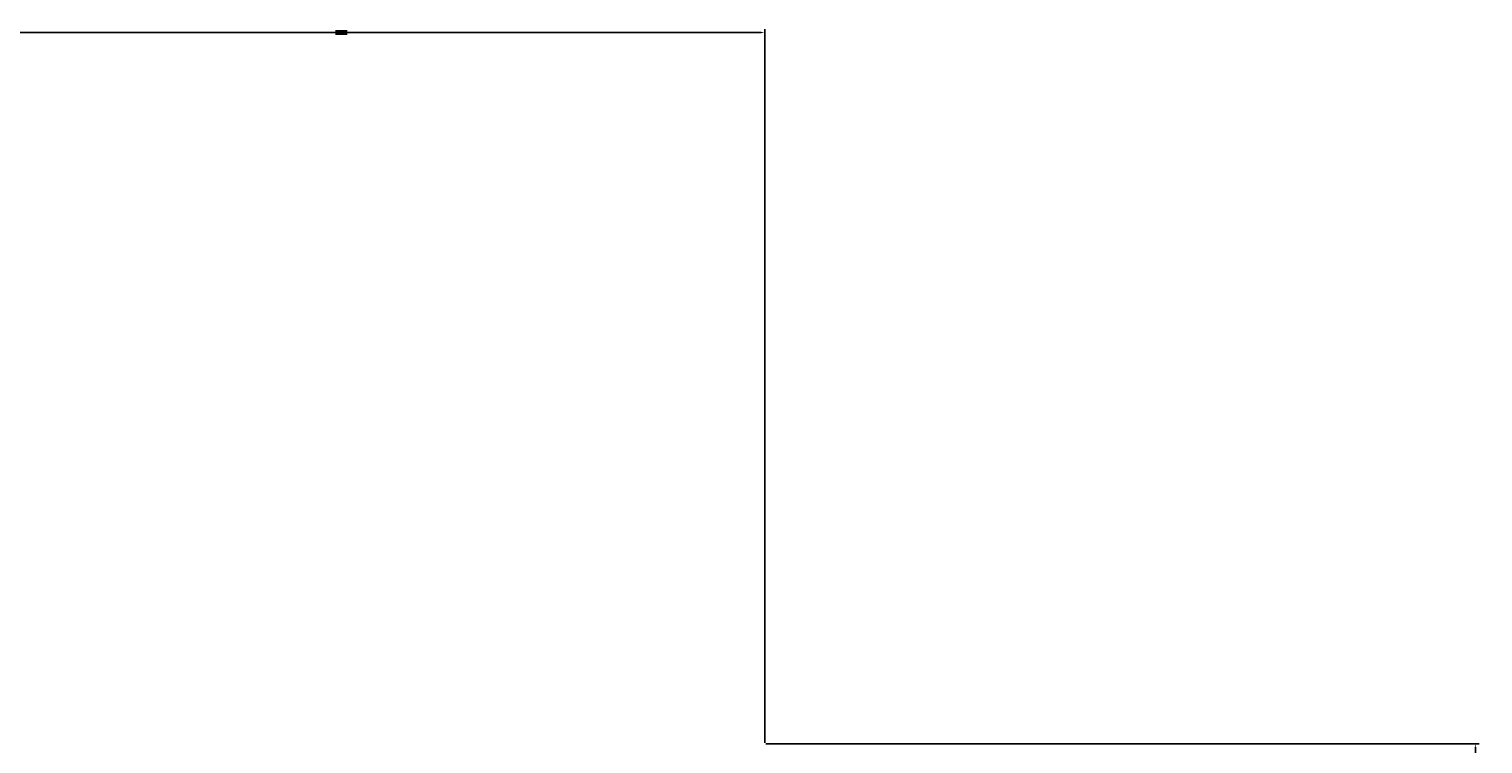
# Model space of a CAD drawing. Units: inches. Extents: x -128 to 854, y -395 to 398.
# Tile 50 of 61: x 275 to 352, y 349 to 387. Entities that reach past the tile are written whole.
import ezdxf

# ---------------------------------------------------------------- set-up
doc = ezdxf.new("R2010")
doc.units = ezdxf.units.IN
doc.header["$MEASUREMENT"] = 0
doc.layers.add('A-ANNO-DIMS', color=2, linetype='Continuous', lineweight=18)
doc.styles.get("Standard").update_dxf_attribs({"font": 'arial.ttf'})
doc.dimstyles.get("Standard").update_dxf_attribs({"dimtxt": 0.18, "dimasz": 0.18, "dimexe": 0.18, "dimexo": 0.0625, "dimgap": 0.09, "dimtad": 0, "dimtih": 1, "dimtoh": 1, "dimdec": 1, "dimzin": 0, "dimdsep": 46, "dimlunit": 4, "dimtxsty": 'Standard', "dimcen": 0.09, "dimclrd": 1, "dimclre": 2, "dimclrt": 6, "dimadec": 0, "dimazin": 0, "dimtfac": 1, "dimtdec": 1, "dimtofl": 0, "dimtmove": 0, "dimatfit": 3, "dimfxl": 1, "dimtfill": 2, "dimtfillclr": 3, "dimtolj": 1, "dimtzin": 0, "dimarcsym": 0})

# ---------------------------------------------------------------- blocks, each defined once
blk = doc.blocks.new('*D97')
at = {"layer": 'A-ANNO-DIMS', "color": 2, "lineweight": -2, "transparency": 16777216}
for p, q in [((-50.127, 348.803), (-50.127, 386.743)), ((313.873, 348.803), (313.873, 386.743))]:
    blk.add_line(p, q, dxfattribs=at)
at = {"layer": 'A-ANNO-DIMS', "color": 1, "lineweight": -2, "transparency": 16777216}
for p, q in [((-49.947, 386.563), (131.474, 386.563)), ((313.693, 386.563), (132.272, 386.563))]:
    blk.add_line(p, q, dxfattribs=at)
at = {"layer": 'A-ANNO-DIMS', "color": 1, "transparency": 16777216}
for points in [[(-49.947, 386.593), (-49.947, 386.533), (-50.127, 386.563)], [(313.693, 386.593), (313.693, 386.533), (313.873, 386.563)]]:
    blk.add_solid(points, dxfattribs=at)
at = {"layer": 'Defpoints', "color": 0, "transparency": 16777216}
for p in [(313.873, 386.563), (-50.127, 348.741), (313.873, 348.741)]:
    blk.add_point(p, dxfattribs=at)
at = {"layer": 'A-ANNO-DIMS', "color": 6, "transparency": 16777216, "insert": (131.873, 386.563), "char_height": 0.18, "attachment_point": 5, "bg_fill": 1, "box_fill_scale": 1.25, "bg_fill_color": 3, "bg_fill_transparency": 0}
blk.add_mtext('\\A1;30\'-4"', dxfattribs=at)
blk = doc.blocks.new('*D98')
at = {"layer": 'A-ANNO-DIMS', "color": 2, "lineweight": -2, "transparency": 16777216}
for p, q in [((313.935, 348.741), (351.853, 348.741)), ((313.935, -89.259), (351.853, -89.259))]:
    blk.add_line(p, q, dxfattribs=at)
at = {"layer": 'A-ANNO-DIMS', "color": 1, "lineweight": -2, "transparency": 16777216}
for p, q in [((351.673, 348.561), (351.673, 129.923)), ((351.673, -89.079), (351.673, 129.559))]:
    blk.add_line(p, q, dxfattribs=at)
at = {"layer": 'A-ANNO-DIMS', "color": 1, "transparency": 16777216}
for points in [[(351.643, 348.561), (351.703, 348.561), (351.673, 348.741)], [(351.643, -89.079), (351.703, -89.079), (351.673, -89.259)]]:
    blk.add_solid(points, dxfattribs=at)
at = {"layer": 'Defpoints', "color": 0, "transparency": 16777216}
for p in [(313.873, 348.741), (351.673, 348.741), (313.873, -89.259)]:
    blk.add_point(p, dxfattribs=at)
at = {"layer": 'A-ANNO-DIMS', "color": 6, "transparency": 16777216, "insert": (351.673, 129.741), "char_height": 0.18, "attachment_point": 5, "bg_fill": 1, "box_fill_scale": 1.25, "bg_fill_color": 3, "bg_fill_transparency": 0}
blk.add_mtext('\\A1;36\'-6"', dxfattribs=at)
blk = doc.blocks.new('*D105')
at = {"layer": 'A-ANNO-DIMS', "color": 2, "lineweight": -2, "transparency": 16777216}
for p, q in [((268.873, 348.803), (268.873, 386.743)), ((313.873, 348.803), (313.873, 386.743))]:
    blk.add_line(p, q, dxfattribs=at)
at = {"layer": 'A-ANNO-DIMS', "color": 1, "lineweight": -2, "transparency": 16777216}
for p, q in [((269.053, 386.563), (291.044, 386.563)), ((313.693, 386.563), (291.702, 386.563))]:
    blk.add_line(p, q, dxfattribs=at)
at = {"layer": 'A-ANNO-DIMS', "color": 1, "transparency": 16777216}
for points in [[(269.053, 386.593), (269.053, 386.533), (268.873, 386.563)], [(313.693, 386.593), (313.693, 386.533), (313.873, 386.563)]]:
    blk.add_solid(points, dxfattribs=at)
at = {"layer": 'Defpoints', "color": 0, "transparency": 16777216}
for p in [(268.873, 386.563), (268.873, 348.741), (313.873, 348.741)]:
    blk.add_point(p, dxfattribs=at)
at = {"layer": 'A-ANNO-DIMS', "color": 6, "transparency": 16777216, "insert": (291.373, 386.563), "char_height": 0.18, "attachment_point": 5, "bg_fill": 1, "box_fill_scale": 1.25, "bg_fill_color": 3, "bg_fill_transparency": 0}
blk.add_mtext('\\A1;3\'-9"', dxfattribs=at)
blk = doc.blocks.new('*D113')
at = {"layer": 'A-ANNO-DIMS', "color": 2, "lineweight": -2, "transparency": 16777216}
for p, q in [((313.935196, 348.740541), (351.852696, 348.740541)), ((313.935196, 293.740541), (351.852696, 293.740541))]:
    blk.add_line(p, q, dxfattribs=at)
at = {"layer": 'A-ANNO-DIMS', "color": 1, "lineweight": -2, "transparency": 16777216}
for p, q in [((351.672696, 348.560541), (351.672696, 321.420541)), ((351.672696, 293.920541), (351.672696, 321.060541))]:
    blk.add_line(p, q, dxfattribs=at)
at = {"layer": 'A-ANNO-DIMS', "color": 1, "transparency": 16777216}
for points in [[(351.642696, 348.560541), (351.702696, 348.560541), (351.672696, 348.740541)], [(351.642696, 293.920541), (351.702696, 293.920541), (351.672696, 293.740541)]]:
    blk.add_solid(points, dxfattribs=at)
at = {"layer": 'Defpoints', "color": 0, "transparency": 16777216}
for p in [(313.872696, 348.740541), (313.872696, 293.740541), (351.672696, 293.740541)]:
    blk.add_point(p, dxfattribs=at)
at = {"layer": 'A-ANNO-DIMS', "color": 6, "transparency": 16777216, "insert": (351.672696, 321.240541), "char_height": 0.18, "attachment_point": 5, "bg_fill": 1, "box_fill_scale": 1.25, "bg_fill_color": 3, "bg_fill_transparency": 0}
blk.add_mtext('\\A1;4\'-7"', dxfattribs=at)

msp = doc.modelspace()

# ---------------------------------------------------------------- dimensions: what is measured, and where the dimension line sits
at = {"layer": 'A-ANNO-DIMS'}
for base, p1, p2, picture, middle in [((313.873, 386.563), (-50.127, 348.741), (313.873, 348.741), '*D97', (131.873, 386.563)), ((268.873, 386.563), (313.873, 348.741), (268.873, 348.741), '*D105', (291.373, 386.563))]:
    dim = msp.add_linear_dim(base=base, p1=p1, p2=p2, dimstyle='Standard', override={"dimdec": 1, "dimlfac": 1, "dimrnd": 0, "dimzin": 1, "dimdsep": 46, "dimlunit": 4, "dimfrac": 2}, dxfattribs=at)
    dim.commit()
    dim.dimension.update_dxf_attribs({"geometry": picture, "text_midpoint": middle})
for base, p1, p2, picture, middle in [((351.673, 348.741), (313.873, -89.259), (313.873, 348.741), '*D98', (351.673, 129.741)), ((351.673, 293.741), (313.873, 348.741), (313.873, 293.741), '*D113', (351.673, 321.241))]:
    dim = msp.add_linear_dim(base=base, p1=p1, p2=p2, angle=90, dimstyle='Standard', override={"dimdec": 1, "dimlfac": 1, "dimrnd": 0, "dimzin": 1, "dimdsep": 46, "dimlunit": 4, "dimfrac": 2}, dxfattribs=at)
    dim.commit()
    dim.dimension.update_dxf_attribs({"geometry": picture, "text_midpoint": middle})

doc.saveas('drawing.dxf')
